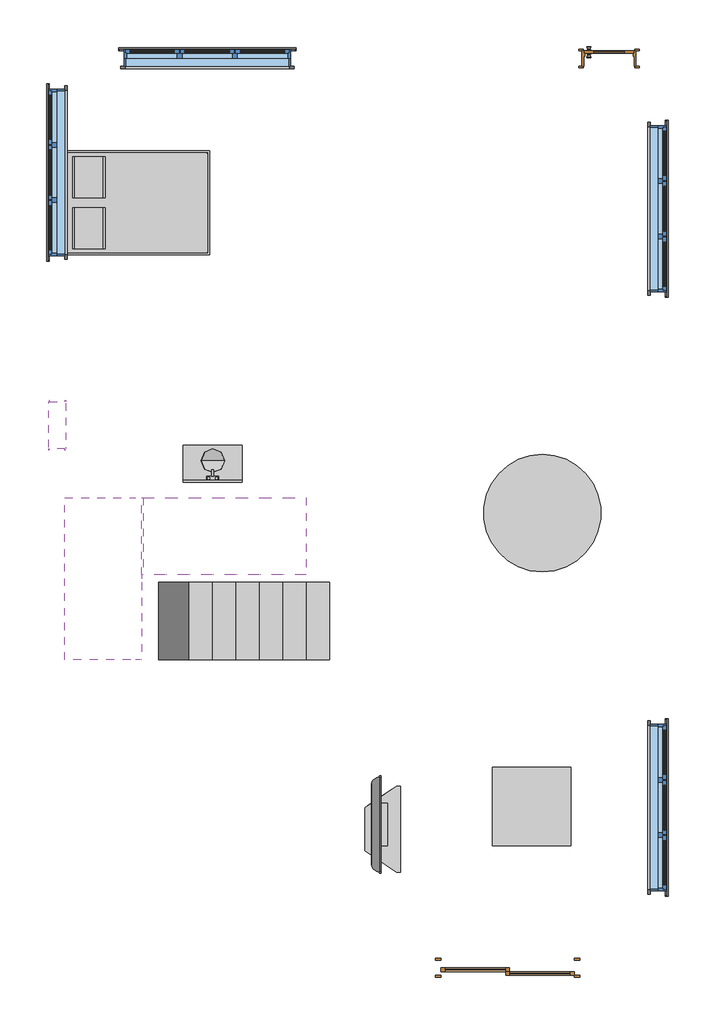
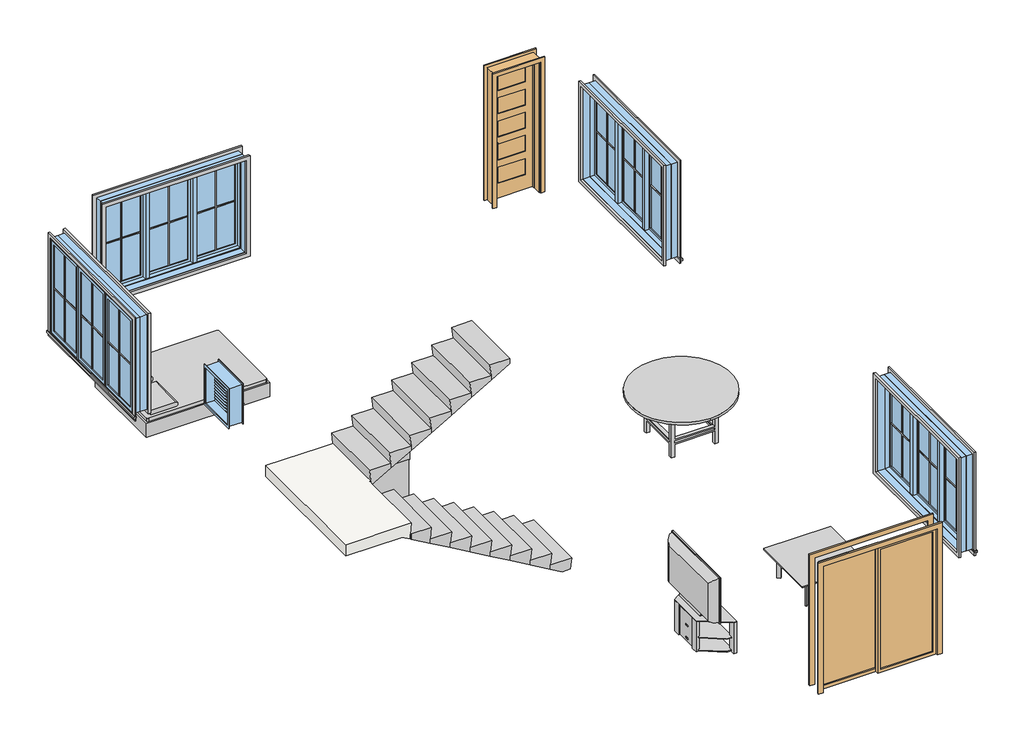
# One storey, incomplete: 20 proxies, 5 furniture elements, 5 windows, 2 doors, 2 stair flights, 1 flow terminal, 1 slab.
"""IFC4 building model written with IfcOpenShell, lengths in millimetres."""

from ifc_helpers import new_model, si_unit, origin, place, context, project, spatial, faceted_brep, transform, mapped, element, save
from components import muntin_pattern_2x2_muntin_pattern_2x2_6849e3ed, muntin_pattern_2x2_muntin_pattern_2x2_a6c43cb1, trim_window_exterior_flat_with_sill_088bf4ff, trim_window_interior_flat_picture_frame_12843d3c, door_e30895c2, door_interior_single_5_panel_vert_wood_650_x_2100_a7f2c8da, flow_terminal_15267b2a, furniture_7b9c1204, furniture_b58f7881, furniture_0b81fedb, tv_stand_tv_stand_6ac32a77, furniture_86cdcdde, window_45599283, window_35a91c22

model = new_model("IFC4")

# Units and contexts
model_context = context("Model", 3, world=origin())
ifc_project = project(units=[si_unit("LENGTHUNIT", "METRE", prefix="MILLI")], contexts=[model_context])

# Site, building, storey
site = spatial("IfcSite", under=ifc_project)
building = spatial("IfcBuilding", under=site)
storey = spatial("IfcBuildingStorey", under=building, Elevation=400.0)

# Proxies
placement = place(None, origin())
muntin_pattern_2x2_muntin_pattern_2x2_shape = muntin_pattern_2x2_muntin_pattern_2x2_6849e3ed(model_context)
element("IfcBuildingElementProxy", 1, Name="Muntin Pattern_2x2 : Muntin Pattern_2x2", ObjectType="Muntin Pattern_2x2 : Muntin Pattern_2x2", at=placement, inside=storey, context=model_context, shape_type="MappedRepresentation", body=[
    mapped(muntin_pattern_2x2_muntin_pattern_2x2_shape, transform((2649.7091997, -1368.0932863, 1083.95), x_axis=(0.0, -1.0, 0.0), y_axis=(1.0, 0.0, 0.0), z_axis=(0.0, 0.0, 1.0))),
])
element("IfcBuildingElementProxy", 2, Name="Muntin Pattern_2x2 : Muntin Pattern_2x2", ObjectType="Muntin Pattern_2x2 : Muntin Pattern_2x2", at=placement, inside=storey, context=model_context, shape_type="MappedRepresentation", body=[
    mapped(muntin_pattern_2x2_muntin_pattern_2x2_shape, transform((-4008.3158003, 7725.3317137, 1058.55), x_axis=(1.0, 0.0, 0.0), y_axis=(0.0, 1.0, 0.0), z_axis=(0.0, 0.0, 1.0))),
])
element("IfcBuildingElementProxy", 3, Name="Muntin Pattern_2x2 : Muntin Pattern_2x2", ObjectType="Muntin Pattern_2x2 : Muntin Pattern_2x2", at=placement, inside=storey, context=model_context, shape_type="MappedRepresentation", body=[
    mapped(muntin_pattern_2x2_muntin_pattern_2x2_shape, transform((-5331.2408003, 5437.8067137, 1058.55), x_axis=(0.0, 1.0, 0.0), y_axis=(-1.0, 0.0, 0.0), z_axis=(0.0, 0.0, 1.0))),
])
element("IfcBuildingElementProxy", 4, Name="Muntin Pattern_2x2 : Muntin Pattern_2x2", ObjectType="Muntin Pattern_2x2 : Muntin Pattern_2x2", at=placement, inside=storey, context=model_context, shape_type="MappedRepresentation", body=[
    mapped(muntin_pattern_2x2_muntin_pattern_2x2_shape, transform((2649.7091997, 6402.4067137, 1071.25), x_axis=(0.0, -1.0, 0.0), y_axis=(1.0, 0.0, 0.0), z_axis=(0.0, 0.0, 1.0))),
])
muntin_pattern_2x2_muntin_pattern_2x2_2_shape = muntin_pattern_2x2_muntin_pattern_2x2_a6c43cb1(model_context)
element("IfcBuildingElementProxy", 5, Name="Muntin Pattern_2x2 : Muntin Pattern_2x2", ObjectType="Muntin Pattern_2x2 : Muntin Pattern_2x2", at=placement, inside=storey, context=model_context, shape_type="MappedRepresentation", body=[
    mapped(muntin_pattern_2x2_muntin_pattern_2x2_2_shape, transform((2649.7091997, -2803.1932863, 1083.95), x_axis=(0.0, 1.0, 0.0), y_axis=(-1.0, 0.0, 0.0), z_axis=(0.0, 0.0, 1.0))),
])
element("IfcBuildingElementProxy", 6, Name="Muntin Pattern_2x2 : Muntin Pattern_2x2", ObjectType="Muntin Pattern_2x2 : Muntin Pattern_2x2", at=placement, inside=storey, context=model_context, shape_type="MappedRepresentation", body=[
    mapped(muntin_pattern_2x2_muntin_pattern_2x2_2_shape, transform((2649.7091997, -2085.6432863, 1083.95), x_axis=(0.0, 1.0, 0.0), y_axis=(-1.0, 0.0, 0.0), z_axis=(0.0, 0.0, 1.0))),
])
element("IfcBuildingElementProxy", 7, Name="Muntin Pattern_2x2 : Muntin Pattern_2x2", ObjectType="Muntin Pattern_2x2 : Muntin Pattern_2x2", at=placement, inside=storey, context=model_context, shape_type="MappedRepresentation", body=[
    mapped(muntin_pattern_2x2_muntin_pattern_2x2_2_shape, transform((-2573.2158003, 7725.3317137, 1058.55), x_axis=(-1.0, 0.0, 0.0), y_axis=(0.0, -1.0, 0.0), z_axis=(0.0, 0.0, 1.0))),
])
element("IfcBuildingElementProxy", 8, Name="Muntin Pattern_2x2 : Muntin Pattern_2x2", ObjectType="Muntin Pattern_2x2 : Muntin Pattern_2x2", at=placement, inside=storey, context=model_context, shape_type="MappedRepresentation", body=[
    mapped(muntin_pattern_2x2_muntin_pattern_2x2_2_shape, transform((-3290.7658003, 7725.3317137, 1058.55), x_axis=(-1.0, 0.0, 0.0), y_axis=(0.0, -1.0, 0.0), z_axis=(0.0, 0.0, 1.0))),
])
element("IfcBuildingElementProxy", 9, Name="Muntin Pattern_2x2 : Muntin Pattern_2x2", ObjectType="Muntin Pattern_2x2 : Muntin Pattern_2x2", at=placement, inside=storey, context=model_context, shape_type="MappedRepresentation", body=[
    mapped(muntin_pattern_2x2_muntin_pattern_2x2_2_shape, transform((-5331.2408003, 6872.9067137, 1058.55), x_axis=(0.0, -1.0, 0.0), y_axis=(1.0, 0.0, 0.0), z_axis=(0.0, 0.0, 1.0))),
])
element("IfcBuildingElementProxy", 10, Name="Muntin Pattern_2x2 : Muntin Pattern_2x2", ObjectType="Muntin Pattern_2x2 : Muntin Pattern_2x2", at=placement, inside=storey, context=model_context, shape_type="MappedRepresentation", body=[
    mapped(muntin_pattern_2x2_muntin_pattern_2x2_2_shape, transform((-5331.2408003, 6155.3567137, 1058.55), x_axis=(0.0, -1.0, 0.0), y_axis=(1.0, 0.0, 0.0), z_axis=(0.0, 0.0, 1.0))),
])
element("IfcBuildingElementProxy", 11, Name="Muntin Pattern_2x2 : Muntin Pattern_2x2", ObjectType="Muntin Pattern_2x2 : Muntin Pattern_2x2", at=placement, inside=storey, context=model_context, shape_type="MappedRepresentation", body=[
    mapped(muntin_pattern_2x2_muntin_pattern_2x2_2_shape, transform((2649.7091997, 4967.3067137, 1071.25), x_axis=(0.0, 1.0, 0.0), y_axis=(-1.0, 0.0, 0.0), z_axis=(0.0, 0.0, 1.0))),
])
element("IfcBuildingElementProxy", 12, Name="Muntin Pattern_2x2 : Muntin Pattern_2x2", ObjectType="Muntin Pattern_2x2 : Muntin Pattern_2x2", at=placement, inside=storey, context=model_context, shape_type="MappedRepresentation", body=[
    mapped(muntin_pattern_2x2_muntin_pattern_2x2_2_shape, transform((2649.7091997, 5684.8567137, 1071.25), x_axis=(0.0, 1.0, 0.0), y_axis=(-1.0, 0.0, 0.0), z_axis=(0.0, 0.0, 1.0))),
])
trim_window_exterior_flat_with_sill_shape = trim_window_exterior_flat_with_sill_088bf4ff(model_context)
element("IfcBuildingElementProxy", 13, Name="Trim-Window-Exterior-Flat : with Sill", ObjectType="Trim-Window-Exterior-Flat : with Sill", at=placement, inside=storey, context=model_context, shape_type="MappedRepresentation", body=[
    mapped(trim_window_exterior_flat_with_sill_shape, transform((2659.2341997, -2085.6432863, 2538.1), x_axis=(0.0, 1.0, 0.0), y_axis=(0.0, 0.0, 1.0), z_axis=(1.0, 0.0, 0.0))),
])
element("IfcBuildingElementProxy", 14, Name="Trim-Window-Exterior-Flat : with Sill", ObjectType="Trim-Window-Exterior-Flat : with Sill", at=placement, inside=storey, context=model_context, shape_type="MappedRepresentation", body=[
    mapped(trim_window_exterior_flat_with_sill_shape, transform((-3290.7658003, 7734.8567137, 2512.7), x_axis=(-1.0, 0.0, 0.0), y_axis=(0.0, 0.0, 1.0), z_axis=(0.0, 1.0, 0.0))),
])
element("IfcBuildingElementProxy", 15, Name="Trim-Window-Exterior-Flat : with Sill", ObjectType="Trim-Window-Exterior-Flat : with Sill", at=placement, inside=storey, context=model_context, shape_type="MappedRepresentation", body=[
    mapped(trim_window_exterior_flat_with_sill_shape, transform((-5340.7658003, 6155.3567137, 2512.7), x_axis=(0.0, -1.0, 0.0), y_axis=(0.0, 0.0, 1.0), z_axis=(-1.0, 0.0, 0.0))),
])
element("IfcBuildingElementProxy", 16, Name="Trim-Window-Exterior-Flat : with Sill", ObjectType="Trim-Window-Exterior-Flat : with Sill", at=placement, inside=storey, context=model_context, shape_type="MappedRepresentation", body=[
    mapped(trim_window_exterior_flat_with_sill_shape, transform((2659.2341997, 5684.8567137, 2525.4), x_axis=(0.0, 1.0, 0.0), y_axis=(0.0, 0.0, 1.0), z_axis=(1.0, 0.0, 0.0))),
])
trim_window_interior_flat_picture_frame_shape = trim_window_interior_flat_picture_frame_12843d3c(model_context)
element("IfcBuildingElementProxy", 17, Name="Trim-Window-Interior-Flat : Picture Frame", ObjectType="Trim-Window-Interior-Flat : Picture Frame", at=placement, inside=storey, context=model_context, shape_type="MappedRepresentation", body=[
    mapped(trim_window_interior_flat_picture_frame_shape, transform((2459.2341997, -2085.6432863, 2538.1), x_axis=(0.0, -1.0, 0.0), y_axis=(0.0, 0.0, 1.0), z_axis=(-1.0, 0.0, 0.0))),
])
element("IfcBuildingElementProxy", 18, Name="Trim-Window-Interior-Flat : Picture Frame", ObjectType="Trim-Window-Interior-Flat : Picture Frame", at=placement, inside=storey, context=model_context, shape_type="MappedRepresentation", body=[
    mapped(trim_window_interior_flat_picture_frame_shape, transform((-3290.7658003, 7534.8567137, 2512.7), x_axis=(1.0, 0.0, 0.0), y_axis=(0.0, 0.0, 1.0), z_axis=(0.0, -1.0, 0.0))),
])
element("IfcBuildingElementProxy", 19, Name="Trim-Window-Interior-Flat : Picture Frame", ObjectType="Trim-Window-Interior-Flat : Picture Frame", at=placement, inside=storey, context=model_context, shape_type="MappedRepresentation", body=[
    mapped(trim_window_interior_flat_picture_frame_shape, transform((-5140.7658003, 6155.3567137, 2512.7), x_axis=(0.0, 1.0, 0.0), y_axis=(0.0, 0.0, 1.0), z_axis=(1.0, 0.0, 0.0))),
])
element("IfcBuildingElementProxy", 20, Name="Trim-Window-Interior-Flat : Picture Frame", ObjectType="Trim-Window-Interior-Flat : Picture Frame", at=placement, inside=storey, context=model_context, shape_type="MappedRepresentation", body=[
    mapped(trim_window_interior_flat_picture_frame_shape, transform((2459.2341997, 5684.8567137, 2525.4), x_axis=(0.0, -1.0, 0.0), y_axis=(0.0, 0.0, 1.0), z_axis=(-1.0, 0.0, 0.0))),
])

# Doors
door_shape = door_e30895c2(model_context)
element("IfcDoor", 21, ObjectType="Door-Double-Sliding : 68\" x 80\"", at=placement, inside=storey, context=model_context, shape_type="MappedRepresentation", body=[
    mapped(door_shape, transform((609.2341997, -4038.1432863, 400.0), x_axis=(-1.0, 0.0, 0.0), y_axis=(0.0, -1.0, 0.0), z_axis=(0.0, 0.0, 1.0))),
])
door_interior_single_5_panel_vert_wood_650_x_2100_shape = door_interior_single_5_panel_vert_wood_650_x_2100_a7f2c8da(model_context)
element("IfcDoor", 22, ObjectType="Door-Interior-Single-5_Panel_Vert-Wood : 650 x 2100", at=placement, inside=storey, context=model_context, shape_type="MappedRepresentation", body=[
    mapped(door_interior_single_5_panel_vert_wood_650_x_2100_shape, transform((1926.6341997, 7638.0317137, 400.0), x_axis=(1.0, 0.0, 0.0), y_axis=(0.0, 1.0, 0.0), z_axis=(0.0, 0.0, 1.0))),
])

# Flow terminal
flow_terminal_shape = flow_terminal_15267b2a(model_context)
element("IfcFlowTerminal", 23, ObjectType="Lavatory - Vanity : 30\"x18\" - Public", at=placement, inside=storey, context=model_context, shape_type="MappedRepresentation", body=[
    mapped(flow_terminal_shape, transform((-3220.7658003, 2134.8567137, 400.0), x_axis=(0.0, 1.0, 0.0), y_axis=(-1.0, 0.0, 0.0), z_axis=(0.0, 0.0, 1.0))),
])

# Furniture
furniture_shape = furniture_7b9c1204(model_context)
element("IfcFurniture", 24, ObjectType="40\" x 40\"", at=placement, inside=storey, context=model_context, shape_type="MappedRepresentation", body=[
    mapped(furniture_shape, transform((976.4145276, -2013.1826305, 400.0), x_axis=(1.0, 0.0, 0.0), y_axis=(0.0, 1.0, 0.0), z_axis=(0.0, 0.0, 1.0))),
])
furniture_2_shape = furniture_b58f7881(model_context)
element("IfcFurniture", 25, ObjectType="Bed-Box : Double 53\" x 74\"", at=placement, inside=storey, context=model_context, shape_type="MappedRepresentation", body=[
    mapped(furniture_2_shape, transform((-4435.3953085, 5422.6042547, 400.0), x_axis=(0.0, 1.0, 0.0), y_axis=(-1.0, 0.0, 0.0), z_axis=(0.0, 0.0, 1.0))),
])
furniture_3_shape = furniture_0b81fedb(model_context)
element("IfcFurniture", 26, ObjectType="TV - Flat Screen : 50\"", at=placement, inside=storey, context=model_context, shape_type="MappedRepresentation", body=[
    mapped(furniture_3_shape, transform((-1103.2444834, -2301.1987721, 900.0), x_axis=(0.0, 1.0, 0.0), y_axis=(-1.0, 0.0, 0.0), z_axis=(0.0, 0.0, 1.0))),
])
tv_stand_tv_stand_shape = tv_stand_tv_stand_6ac32a77(model_context)
element("IfcFurniture", 27, ObjectType="TV Stand : TV Stand", at=placement, inside=storey, context=model_context, shape_type="MappedRepresentation", body=[
    mapped(tv_stand_tv_stand_shape, transform((-1240.7658003, -2490.3312883, 400.0), x_axis=(0.0, 1.0, 0.0), y_axis=(-1.0, 0.0, 0.0), z_axis=(0.0, 0.0, 1.0))),
])
furniture_4_shape = furniture_86cdcdde(model_context)
element("IfcFurniture", 28, ObjectType="Table-Dining Round w Chairs : 60\" Diameter", at=placement, inside=storey, context=model_context, shape_type="MappedRepresentation", body=[
    mapped(furniture_4_shape, transform((955.5522325, 1919.7354023, 400.0), x_axis=(1.0, 0.0, 0.0), y_axis=(0.0, 1.0, 0.0), z_axis=(0.0, 0.0, 1.0))),
])

# Slab
element("IfcSlab", 29, ObjectType="7\" Thickness", at=placement, inside=storey, context=model_context, shape_type="Brep", body=[
    faceted_brep([(-4140.7658003, 834.8567137, 1988.2352941), (-4140.7658003, -165.1432863, 1988.2352941), (-4159.8158003, -165.1432863, 1811.7647059), (-4159.8158003, 834.8567137, 1811.7647059), (-4140.7658003, 934.8567137, 1988.2352941), (-4121.7158003, 934.8567137, 1988.2352941), (-4121.7158003, 1934.8567137, 1988.2352941), (-4140.7658003, 1934.8567137, 1988.2352941), (-4302.0786253, 1934.8567137, 1988.2352941), (-5140.7658003, 1934.8567137, 1988.2352941), (-5140.7658003, -165.1432863, 1988.2352941), (-4284.2529753, -165.1432863, 1988.2352941), (-4159.8158003, -165.1432863, 1738.3896856), (-4159.8158003, 834.8567137, 1738.3896856), (-4159.8158003, 834.8567137, 1810.4352941), (-4140.7658003, 834.8567137, 1810.4352941), (-4140.7658003, 934.8567137, 1810.4352941), (-4140.7658003, 934.8567137, 1903.8308621), (-4121.7158003, 934.8567137, 1914.8602739), (-4121.7158003, 1934.8567137, 1914.8602739), (-4140.7658003, 1934.8567137, 1903.8308621), (-4302.0786253, 1934.8567137, 1810.4352941), (-5140.7658003, 1934.8567137, 1810.4352941), (-5140.7658003, -165.1432863, 1810.4352941), (-4284.2529753, -165.1432863, 1810.4352941), (-4302.0786253, 934.8567137, 1810.4352941), (-4284.2529753, 834.8567137, 1810.4352941)], [[[0, 1, 2, 3]], [[0, 4, 5, 6, 7, 8, 9, 10, 11, 1]], [[3, 2, 12, 13, 14]], [[0, 3, 14, 15]], [[4, 0, 15, 16, 17]], [[5, 4, 17, 18]], [[6, 5, 18, 19]], [[7, 6, 19, 20]], [[7, 20, 21, 22, 9, 8]], [[10, 9, 22, 23]], [[2, 1, 11, 10, 23, 24, 12]], [[25, 16, 15, 14, 26, 24, 23, 22, 21]], [[16, 25, 17]], [[24, 26, 13, 12]], [[26, 14, 13]], [[25, 21, 20, 19, 18, 17]]]),
])

# Stair flights
element("IfcStairFlight", 30, ObjectType="3/4\" Nosing", at=placement, inside=storey, context=model_context, shape_type="Brep", body=[
    faceted_brep([(-1702.3658003, 834.8567137, 576.4705882), (-1702.3658003, -165.1432863, 576.4705882), (-1721.4158003, -165.1432863, 400.0), (-1721.4158003, 834.8567137, 400.0), (-2026.2158003, 834.8567137, 576.4705882), (-2026.2158003, -165.1432863, 576.4705882), (-2026.2158003, -165.1432863, 503.095568), (-1848.1491353, -165.1432863, 400.0), (-1848.1491353, 834.8567137, 400.0), (-2026.2158003, 834.8567137, 503.095568), (-2007.1658003, -165.1432863, 752.9411765), (-2007.1658003, 834.8567137, 752.9411765), (-2331.0158003, 834.8567137, 752.9411765), (-2331.0158003, -165.1432863, 752.9411765), (-2331.0158003, -165.1432863, 679.5661562), (-2331.0158003, 834.8567137, 679.5661562), (-2311.9658003, -165.1432863, 929.4117647), (-2311.9658003, 834.8567137, 929.4117647), (-2635.8158003, 834.8567137, 929.4117647), (-2635.8158003, -165.1432863, 929.4117647), (-2635.8158003, -165.1432863, 856.0367444), (-2635.8158003, 834.8567137, 856.0367444), (-2616.7658003, -165.1432863, 1105.8823529), (-2616.7658003, 834.8567137, 1105.8823529), (-2940.6158003, 834.8567137, 1105.8823529), (-2940.6158003, -165.1432863, 1105.8823529), (-2940.6158003, -165.1432863, 1032.5073327), (-2940.6158003, 834.8567137, 1032.5073327), (-2921.5658003, -165.1432863, 1282.3529412), (-2921.5658003, 834.8567137, 1282.3529412), (-3245.4158003, 834.8567137, 1282.3529412), (-3245.4158003, -165.1432863, 1282.3529412), (-3245.4158003, -165.1432863, 1208.9779209), (-3245.4158003, 834.8567137, 1208.9779209), (-3226.3658003, -165.1432863, 1458.8235294), (-3226.3658003, 834.8567137, 1458.8235294), (-3550.2158003, 834.8567137, 1458.8235294), (-3550.2158003, -165.1432863, 1458.8235294), (-3550.2158003, -165.1432863, 1385.4485091), (-3550.2158003, 834.8567137, 1385.4485091), (-3531.1658003, -165.1432863, 1635.2941176), (-3531.1658003, 834.8567137, 1635.2941176), (-3855.0158003, 834.8567137, 1635.2941176), (-3855.0158003, -165.1432863, 1635.2941176), (-3855.0158003, -165.1432863, 1561.9190974), (-3855.0158003, 834.8567137, 1561.9190974), (-4159.8158003, -165.1432863, 1811.7647059), (-4140.7658003, -165.1432863, 1811.7647059), (-3835.9658003, -165.1432863, 1811.7647059), (-3835.9658003, 834.8567137, 1811.7647059), (-4140.7658003, 834.8567137, 1811.7647059), (-4159.8158003, 834.8567137, 1811.7647059), (-4159.8158003, -165.1432863, 1738.3896856), (-4140.7658003, -165.1432863, 1727.3602739), (-4159.8158003, 834.8567137, 1738.3896856), (-4159.8158003, 834.8567137, 1810.4352941)], [[[0, 1, 2, 3]], [[1, 0, 4, 5]], [[1, 5, 6, 7, 2]], [[4, 0, 3, 8, 9]], [[10, 11, 12, 13]], [[10, 13, 14, 6, 5]], [[12, 11, 4, 9, 15]], [[5, 4, 11, 10]], [[16, 17, 18, 19]], [[16, 19, 20, 14, 13]], [[18, 17, 12, 15, 21]], [[13, 12, 17, 16]], [[22, 23, 24, 25]], [[22, 25, 26, 20, 19]], [[24, 23, 18, 21, 27]], [[19, 18, 23, 22]], [[28, 29, 30, 31]], [[28, 31, 32, 26, 25]], [[30, 29, 24, 27, 33]], [[25, 24, 29, 28]], [[34, 35, 36, 37]], [[34, 37, 38, 32, 31]], [[36, 35, 30, 33, 39]], [[31, 30, 35, 34]], [[40, 41, 42, 43]], [[40, 43, 44, 38, 37]], [[42, 41, 36, 39, 45]], [[37, 36, 41, 40]], [[46, 47, 48, 49, 50, 51]], [[47, 46, 52, 53]], [[49, 42, 45, 54, 55, 51, 50]], [[46, 51, 55, 54, 52]], [[43, 42, 49, 48]], [[3, 2, 7, 8]], [[8, 7, 6, 14, 20, 26, 32, 38, 44, 53, 52, 54, 45, 39, 33, 27, 21, 15, 9]], [[48, 47, 53, 44, 43]]]),
])
element("IfcStairFlight", 31, ObjectType="3/4\" Nosing", at=placement, inside=storey, context=model_context, shape_type="Brep", body=[
    faceted_brep([(-4140.7658003, 934.8567137, 2164.7058824), (-4140.7658003, 1934.8567137, 2164.7058824), (-4121.7158003, 1934.8567137, 1988.2352941), (-4121.7158003, 934.8567137, 1988.2352941), (-3816.9158003, 934.8567137, 2164.7058824), (-3816.9158003, 1934.8567137, 2164.7058824), (-3816.9158003, 1934.8567137, 2091.3308621), (-4121.7158003, 1934.8567137, 1914.8602739), (-4121.7158003, 934.8567137, 1914.8602739), (-3816.9158003, 934.8567137, 2091.3308621), (-3835.9658003, 1934.8567137, 2341.1764706), (-3835.9658003, 934.8567137, 2341.1764706), (-3512.1158003, 934.8567137, 2341.1764706), (-3512.1158003, 1934.8567137, 2341.1764706), (-3512.1158003, 1934.8567137, 2267.8014503), (-3512.1158003, 934.8567137, 2267.8014503), (-3531.1658003, 1934.8567137, 2517.6470588), (-3531.1658003, 934.8567137, 2517.6470588), (-3207.3158003, 934.8567137, 2517.6470588), (-3207.3158003, 1934.8567137, 2517.6470588), (-3207.3158003, 1934.8567137, 2444.2720386), (-3207.3158003, 934.8567137, 2444.2720386), (-3226.3658003, 1934.8567137, 2694.1176471), (-3226.3658003, 934.8567137, 2694.1176471), (-2902.5158003, 934.8567137, 2694.1176471), (-2902.5158003, 1934.8567137, 2694.1176471), (-2902.5158003, 1934.8567137, 2620.7426268), (-2902.5158003, 934.8567137, 2620.7426268), (-2921.5658003, 1934.8567137, 2870.5882353), (-2921.5658003, 934.8567137, 2870.5882353), (-2597.7158003, 934.8567137, 2870.5882353), (-2597.7158003, 1934.8567137, 2870.5882353), (-2597.7158003, 1934.8567137, 2797.213215), (-2597.7158003, 934.8567137, 2797.213215), (-2616.7658003, 1934.8567137, 3047.0588235), (-2616.7658003, 934.8567137, 3047.0588235), (-2292.9158003, 934.8567137, 3047.0588235), (-2292.9158003, 1934.8567137, 3047.0588235), (-2292.9158003, 1934.8567137, 2973.6838033), (-2292.9158003, 934.8567137, 2973.6838033), (-2311.9658003, 1934.8567137, 3223.5294118), (-2311.9658003, 934.8567137, 3223.5294118), (-2007.1658003, 934.8567137, 3223.5294118), (-2007.1658003, 1934.8567137, 3223.5294118), (-2007.1658003, 1934.8567137, 3139.1249797), (-2007.1658003, 934.8567137, 3139.1249797)], [[[0, 1, 2, 3]], [[1, 0, 4, 5]], [[1, 5, 6, 7, 2]], [[3, 2, 7, 8]], [[4, 0, 3, 8, 9]], [[10, 11, 12, 13]], [[10, 13, 14, 6, 5]], [[12, 11, 4, 9, 15]], [[11, 10, 5, 4]], [[16, 17, 18, 19]], [[16, 19, 20, 14, 13]], [[18, 17, 12, 15, 21]], [[17, 16, 13, 12]], [[22, 23, 24, 25]], [[22, 25, 26, 20, 19]], [[24, 23, 18, 21, 27]], [[23, 22, 19, 18]], [[28, 29, 30, 31]], [[28, 31, 32, 26, 25]], [[30, 29, 24, 27, 33]], [[29, 28, 25, 24]], [[34, 35, 36, 37]], [[34, 37, 38, 32, 31]], [[36, 35, 30, 33, 39]], [[35, 34, 31, 30]], [[40, 41, 42, 43]], [[40, 43, 44, 38, 37]], [[42, 41, 36, 39, 45]], [[43, 42, 45, 44]], [[41, 40, 37, 36]], [[7, 6, 14, 20, 26, 32, 38, 44, 45, 39, 33, 27, 21, 15, 9, 8]]]),
])

# Windows
window_shape = window_45599283(model_context)
element("IfcWindow", 32, ObjectType="Window-Casement-Triple : 85\" x 60\"", at=placement, inside=storey, context=model_context, shape_type="MappedRepresentation", body=[
    mapped(window_shape, transform((2559.2341997, -2085.6432863, 99.7), x_axis=(0.0, -1.0, 0.0), y_axis=(1.0, 0.0, 0.0), z_axis=(0.0, 0.0, 1.0))),
])
element("IfcWindow", 33, ObjectType="Window-Casement-Triple : 85\" x 60\"", at=placement, inside=storey, context=model_context, shape_type="MappedRepresentation", body=[
    mapped(window_shape, transform((-3290.7658003, 7634.8567137, 74.3), x_axis=(1.0, 0.0, 0.0), y_axis=(0.0, 1.0, 0.0), z_axis=(0.0, 0.0, 1.0))),
])
element("IfcWindow", 34, ObjectType="Window-Casement-Triple : 85\" x 60\"", at=placement, inside=storey, context=model_context, shape_type="MappedRepresentation", body=[
    mapped(window_shape, transform((-5240.7658003, 6155.3567137, 74.3), x_axis=(0.0, 1.0, 0.0), y_axis=(-1.0, 0.0, 0.0), z_axis=(0.0, 0.0, 1.0))),
])
element("IfcWindow", 35, ObjectType="Window-Casement-Triple : 85\" x 60\"", at=placement, inside=storey, context=model_context, shape_type="MappedRepresentation", body=[
    mapped(window_shape, transform((2559.2341997, 5684.8567137, 87.0), x_axis=(0.0, -1.0, 0.0), y_axis=(1.0, 0.0, 0.0), z_axis=(0.0, 0.0, 1.0))),
])
window_2_shape = window_35a91c22(model_context)
element("IfcWindow", 36, ObjectType="Window-Louvers : 24\" x 24\"", at=placement, inside=storey, context=model_context, shape_type="MappedRepresentation", body=[
    mapped(window_2_shape, transform((-5234.4158003, 2875.3317137, 1385.6), x_axis=(0.0, -1.0, 0.0), y_axis=(1.0, 0.0, 0.0), z_axis=(0.0, 0.0, 1.0))),
])

save(model, "model.ifc")

# Revit data of these elements
# Type "Muntin Pattern_2x2 : Muntin Pattern_2x2"
#   Width [instance default] = 4' - 0"
#   Thickness = 0' - 0 1/2"
#   Height [instance default] = 4' - 0"
#   Distance = 0' - 0 3/4"
#   Interior Material [instance default] = none
#   Exterior Material [instance default] = none
#   Default Elevation = 0
# Type "Trim-Window-Exterior-Flat : with Sill"
#   Trim Width = 0' - 2 1/4"
#   Trim Thickness_Picture Frame = 0' - 1 1/4"
#   Trim Thickness_with Sill = 0' - 0 3/4"
#   Sill Thickness = 0' - 1 1/4"
#   Opening Width [instance default] = 2' - 0"
#   Opening Height [instance default] = 3' - 0"
#   Default Elevation = 4' - 0"
#   Sill = yes
#   Picture Frame = no
#   Trim Material [instance default] = none
# Type "Trim-Window-Interior-Flat : Picture Frame"
#   Trim Thickness_Picture Frame = 0' - 1 1/4"
#   Trim Width = 0' - 2 1/4"
#   Trim Thickness_with Sill = 0' - 0 3/4"
#   Sill Thickness = 0' - 1 1/4"
#   Opening Width [instance default] = 2' - 0"
#   Opening Height [instance default] = 3' - 0"
#   Default Elevation = 4' - 0"
#   Sill = no
#   Picture Frame = yes
#   Trim Material [instance default] = none
# Type "Door-Double-Sliding : 68\" x 80\""
#   Type Mark = "17"
#   Construction Type Id = "opn-d45"
#   Assembly Code = "C1020"
#   Analytic Construction = "Wood frame, double glass door "
#   Thickness = 0' - 2"
#   Thermal Resistance (R) = 1.8150 (h·ft²·°F)/BTU
#   Heat Transfer Coefficient (U) = 0.5510 BTU/(h·ft²·°F)
#   Height = 6' - 8"
#   Rail Width = 0' - 2"
#   Stiles = 0' - 2"
#   Trim Projection Ext = 0' - 1"
#   Trim Projection Int = 0' - 1"
#   Trim Width = 0' - 3"
#   Width = 5' - 8"
#   Define Thermal Properties by = 1
#   Glazing = Glass
#   Panel Material = Wood - Birch - Solid Stained Light Low Gloss
#   Trim Material = Paint - Sienna
#   Visual Light Transmittance = 0
#   Solar Heat Gain Coefficient = 0
#   Function = (empty or 0)
#   Wall Closure = (empty or 0)
# Type "Door-Interior-Single-5_Panel_Vert-Wood : 650 x 2100"
#   Type Mark = "22"
#   Assembly Code = "C1020300"
#   Analytic Construction = "Wooden"
#   Top Rail = 0' - 4 11/16"
#   Thickness = 0' - 1 3/8"
#   Thermal Resistance (R) = 2.5876 (h·ft²·°F)/BTU
#   Swing Angle [instance default] = 90.00°
#   Stiles = 0' - 4 3/4"
#   Rough Width = 2' - 3.59055"
#   Rough Height = 6' - 11.67717"
#   Intermediate Rail = 0' - 4 1/2"
#   Height = 6' - 10.67717"
#   Width = 2' - 1.59055"
#   Heat Transfer Coefficient (U) = 0.3865 BTU/(h·ft²·°F)
#   Bottom Rail = 0' - 9 1/8"
#   Trim Material = Cherry
#   Panel Material = Cherry
#   Frame Material = Cherry
#   Door Handle Material = Aluminum
#   Visual Light Transmittance = 0
#   Solar Heat Gain Coefficient = 0
#   Wall Closure = (empty or 0)
#   Function = (empty or 0)
# Type "Lavatory - Vanity : 30\"x18\" - Public"
#   Sanitary Radius = 5/8"
#   Sanitary Diameter = 1 1/4"
#   WFU = 1
#   Lavatory Length = 1' - 6"
#   Lavatory Width = 2' - 6"
#   Hot Water Radius = 1/4"
#   Hot Water Diameter = 1/2"
#   Half Lavatory Width = 1' - 3"
#   HWFU = 1.5
#   Flow Pressure [instance default] = 8.00 psi
#   Cold Water Radius = 1/4"
#   Cold Water Diameter = 1/2"
#   CWFU = 1.5
#   Sink Material = none
#   Faucet Material = none
#   Cabinet Top Material = none
#   Cabinet Material = none
#   Default Elevation = 0
# Type "40\" x 40\""
#   Assembly Code = "E2020200"
#   Height = 1' - 5"
#   Length = 3' - 4"
#   Width = 3' - 4"
#   Default Elevation = 0
# Type "Bed-Box : Double 53\" x 74\""
#   Assembly Code = "E2020200"
#   Length = 6' - 2"
#   Width = 4' - 5"
#   Frame Material = Birch
#   Mattress Material = Linen, White
#   Default Elevation = 0
# Type "TV - Flat Screen : 50\""
#   SinAng = 0' - 0.0193"
#   L = 3' - 7.57782"
#   H = 2' - 0.51477"
#   Thickness = 0' - 4.33071"
#   Diagonal = 4' - 2"
#   CosAng = 0' - 0.03431"
#   Stand [instance default] = yes
#   Default Elevation = 0
# Type "TV Stand : TV Stand"
#   Depth = 1' - 6"
#   Width = 3' - 8"
#   Height = 1' - 7 1/2"
#   Finish = Melamine - Gray
#   Default Elevation = 0
# Type "Table-Dining Round w Chairs : 60\" Diameter"
#   Assembly Code = "E2020200"
#   Radius = 2' - 6"
#   Diameter = 5' - 0"
#   Height = 2' - 6"
#   Chairs = 6
#   Base Material = Pine
#   Top Material = Laminate, Linen, Matte
#   Default Elevation = 0
# Type "Window-Casement-Triple : 85\" x 60\""
#   Type Mark = "18"
#   Fire Rating = "0.5h"
#   Assembly Code = "B2020100"
#   Analytic Construction = "Double glazing - domestic"
#   Window Inset [instance default] = 0' - 0"
#   Wall Thickness [instance default] = 0' - 6"
#   Muntin Width = 1' - 11"
#   Visual Light Transmittance = 0.81
#   Thermal Resistance (R) = 1.8146 (h·ft²·°F)/BTU
#   Solar Heat Gain Coefficient = 0.76
#   One Third Width = 2' - 4.33333"
#   Sash Width = 2' - 3 1/2"
#   Rough Width = 7' - 1 1/2"
#   Rough Height = 5' - 0 1/2"
#   Interior Wall Closure [instance default] = 0' - 2 1/4"
#   Height = 5' - 0"
#   Heat Transfer Coefficient (U) = 0.5511 BTU/(h·ft²·°F)
#   Muntin Height = 4' - 6 1/2"
#   Frame Extension [instance default] = 0' - 0 1/4"
#   Exterior Wall Closure [instance default] = 0' - 1 1/4"
#   Extension Jamb [instance default] = 0' - 2 1/4"
#   Default Sill Height = 3' - 0"
#   Width = 7' - 1"
#   Middle Muntin Visibility = yes
#   Side Muntin Visibility = yes
#   Interior Trim Visibility [instance default] = yes
#   Exterior Trim Visibility [instance default] = yes
#   Extension Jamb Visibility [instance default] = yes
#   Muntin Pattern = Muntin Pattern_2x2 : Muntin Pattern_2x2
#   Interior Trim Material = Wood - Stained
#   Interior Trim = Trim-Window-Interior-Flat : Picture Frame
#   Interior Frame Material = Wood - Stained
#   Glass Panel Material = Glass
#   Exterior Trim Material = Clad - White
#   Exterior Trim = Trim-Window-Exterior-Flat : with Sill
#   Exterior Frame Material = Clad - White
#   Wall Closure = (empty or 0)
# Type "Window-Louvers : 24\" x 24\""
#   Type Mark = "21"
#   Construction Type Id = "GSP4R"
#   Assembly Code = "B20"
#   Analytic Construction = "1/8 in Pilkington single glazing"
#   Visual Light Transmittance = 0.9
#   Thermal Resistance (R) = 1.53941 (h·ft²·°F)/BTU
#   Solar Heat Gain Coefficient = 0.78
#   Max Height = 1' - 11.74264"
#   Height = 2' - 0"
#   Heat Transfer Coefficient (U) = 0.6496 BTU/(h·ft²·°F)
#   Blade Width [instance default] = 1' - 10 1/2"
#   Blade Vertical Thickness = 0' - 0.35355"
#   Blade Thickness = 0' - 0 1/4"
#   Blade Spacing = 0' - 1 1/2"
#   Blade Height = 0' - 1.85355"
#   Blade Depth = 0' - 3"
#   Blade Angle = 45.00°
#   Default Sill Height = 3' - 0"
#   Trim Projection_Exterior = 0' - 0 1/2"
#   Trim Projection_Interior = 0' - 0 1/2"
#   Trim Width_Exterior = 0' - 1 1/2"
#   Trim Width_Interior = 0' - 1 1/2"
#   Width = 2' - 0"
#   Max Blade Count = 12
#   Define Thermal Properties by = 1
#   Blade Count = 12
#   Frame Material = Birch
#   Louver Material = Birch
#   Trim Exterior Material = Birch
#   Trim Interior Material = Birch
#   Wall Closure = (empty or 0)
# Elements 1, 2, 3, 4, 5, 6, 7, 8, 9, 10, 11, 12 (IfcBuildingElementProxy, "Muntin Pattern_2x2 : Muntin Pattern_2x2")
#   Width = 1' - 11"
#   Height = 4' - 6 1/2"
#   Interior Material = Wood - Stained
#   Exterior Material = Clad - White
#   Phase Created = New Construction
#   Materials on its faces: "Clad - White", "Wood - Stained"
# Elements 13, 14, 15, 16 (IfcBuildingElementProxy, "Trim-Window-Exterior-Flat : with Sill")
#   Opening Width = 7' - 1"
#   Opening Height = 5' - 0"
#   Trim Material = Clad - White
#   Phase Created = New Construction
#   Materials on its faces: "Clad - White"
# Elements 17, 18, 19, 20 (IfcBuildingElementProxy, "Trim-Window-Interior-Flat : Picture Frame")
#   Opening Width = 7' - 1"
#   Opening Height = 5' - 0"
#   Trim Material = Wood - Stained
#   Phase Created = New Construction
#   Materials on its faces: "Wood - Stained"
# Element 21 (IfcDoor, "Door-Double-Sliding : 68\" x 80\"")
#   Phase Created = New Construction
#   Materials on its faces: "Paint - Sienna", "Wood - Birch - Solid Stained Light Low Gloss", "Glass"
# Element 22 (IfcDoor, "Door-Interior-Single-5_Panel_Vert-Wood : 650 x 2100")
#   Swing Angle = 90.00°
#   Phase Created = New Construction
#   Materials on its faces: "Cherry", "Aluminum"
# Element 23 (IfcFlowTerminal, "Lavatory - Vanity : 30\"x18\" - Public")
#   Mark = "2"
#   Flow Pressure = 8.00 psi
#   Phase Created = New Construction
# Element 24 (IfcFurniture, "40\" x 40\"")
#   Phase Created = New Construction
#   Materials on its faces: "Metal - Steel, Polished", "Glass - Clear, Grey"
# Element 25 (IfcFurniture, "Bed-Box : Double 53\" x 74\"")
#   Phase Created = New Construction
#   Materials on its faces: "Birch", "Linen, White"
# Element 26 (IfcFurniture, "TV - Flat Screen : 50\"")
#   Stand = yes
#   Phase Created = New Construction
#   Materials on its faces: "TV - Black", "TV - Glass", "TV - Screen"
# Element 27 (IfcFurniture, "TV Stand : TV Stand")
#   Phase Created = New Construction
#   Materials on its faces: "Melamine - Gray", "Glass - Shelves"
# Element 28 (IfcFurniture, "Table-Dining Round w Chairs : 60\" Diameter")
#   Phase Created = New Construction
#   Materials on its faces: "Pine", "Laminate, Linen, Matte"
# Element 29 (IfcSlab, "7\" Thickness")
#   Phase Created = New Construction
#   Materials on its faces: "Concrete, Cast-in-Place gray"
# Elements 30, 31 (IfcStairFlight, "3/4\" Nosing")
#   Phase Created = New Construction
#   Materials on its faces: "Concrete, Cast-in-Place gray"
# Element 32 (IfcWindow, "Window-Casement-Triple : 85\" x 60\"")
#   Mark = "1"
#   Window Inset = 0' - 0"
#   Interior Wall Closure = 0' - 2 1/4"
#   Frame Extension = 0' - 0 1/4"
#   Exterior Wall Closure = 0' - 1 1/4"
#   Interior Trim Visibility = yes
#   Exterior Trim Visibility = yes
#   Phase Created = New Construction
#   Materials on its faces: "Wood - Stained", "Glass", "Clad - White"
# Element 33 (IfcWindow, "Window-Casement-Triple : 85\" x 60\"")
#   Mark = "2"
#   Window Inset = 0' - 0"
#   Interior Wall Closure = 0' - 2 1/4"
#   Frame Extension = 0' - 0 1/4"
#   Exterior Wall Closure = 0' - 1 1/4"
#   Interior Trim Visibility = yes
#   Exterior Trim Visibility = yes
#   Phase Created = New Construction
#   Materials on its faces: "Wood - Stained", "Glass", "Clad - White"
# Element 34 (IfcWindow, "Window-Casement-Triple : 85\" x 60\"")
#   Mark = "3"
#   Window Inset = 0' - 0"
#   Interior Wall Closure = 0' - 2 1/4"
#   Frame Extension = 0' - 0 1/4"
#   Exterior Wall Closure = 0' - 1 1/4"
#   Interior Trim Visibility = yes
#   Exterior Trim Visibility = yes
#   Phase Created = New Construction
#   Materials on its faces: "Wood - Stained", "Glass", "Clad - White"
# Element 35 (IfcWindow, "Window-Casement-Triple : 85\" x 60\"")
#   Mark = "6"
#   Window Inset = 0' - 0"
#   Interior Wall Closure = 0' - 2 1/4"
#   Frame Extension = 0' - 0 1/4"
#   Exterior Wall Closure = 0' - 1 1/4"
#   Interior Trim Visibility = yes
#   Exterior Trim Visibility = yes
#   Phase Created = New Construction
#   Materials on its faces: "Wood - Stained", "Glass", "Clad - White"
# Element 36 (IfcWindow, "Window-Louvers : 24\" x 24\"")
#   Mark = "5"
#   Blade Width = 1' - 10 1/2"
#   Phase Created = New Construction
#   Materials on its faces: "Birch"
# Materials
#   "Glass": class "Glass", colour RGB 0 128 192, transparency 0.75, Description = "Soda Lime Glass", Cost = 0
#   "Wood - Birch - Solid Stained Light Low Gloss": class "Wood", colour RGB 210 159 95, transparency 0, Cost = 0
#   "Paint - Sienna": colour RGB 118 70 51, transparency 0, Cost = 0
#   "Cherry": class "Wood", colour RGB 226 177 128, transparency 0, Description = "Prunus Serotina", Cost = 0
#   "Aluminum": class "Metal", colour RGB 247 247 247, transparency 0, Description = "Aluminum 6061", Cost = 0
#   "Birch": class "Wood", colour RGB 224 178 126, transparency 0, Description = "Betula Alleghaniensis", Cost = 0
#   "Linen, White": class "Textile", colour RGB 247 247 239, transparency 0, Description = "Linen, white", Cost = 0
#   "Melamine - Gray": class "Wood", colour RGB 49 49 49, transparency 0
#   "Pine": class "Wood", colour RGB 223 192 134, transparency 0, Description = "Pinus Echinata", Cost = 0
#   "Laminate, Linen, Matte": class "Plastic", colour RGB 249 239 230, transparency 0, Description = "Plastic Laminate - Linen, Matte", Cost = 0
#   "Wood - Stained": class "Wood", colour RGB 224 178 126, transparency 0, Cost = 0
#   "Clad - White": class "Wood", colour RGB 242 242 238, transparency 0, Cost = 0
#   "Metal - Steel, Polished": colour RGB 57 57 57, transparency 0
#   "Glass - Clear, Grey": colour RGB 252 255 255, transparency 0.64
#   "TV - Black": colour RGB 49 49 49, transparency 0
#   "TV - Glass": colour RGB 157 157 157, transparency 0.9
#   "TV - Screen": colour RGB 0 0 0, transparency 0
#   "Glass - Shelves": class "Glass", colour RGB 167 167 167, transparency 0.9
#   "Concrete, Cast-in-Place gray": class "Concrete", colour RGB 192 192 192, transparency 0, Description = "Cast-in-place concrete", Cost = 0
